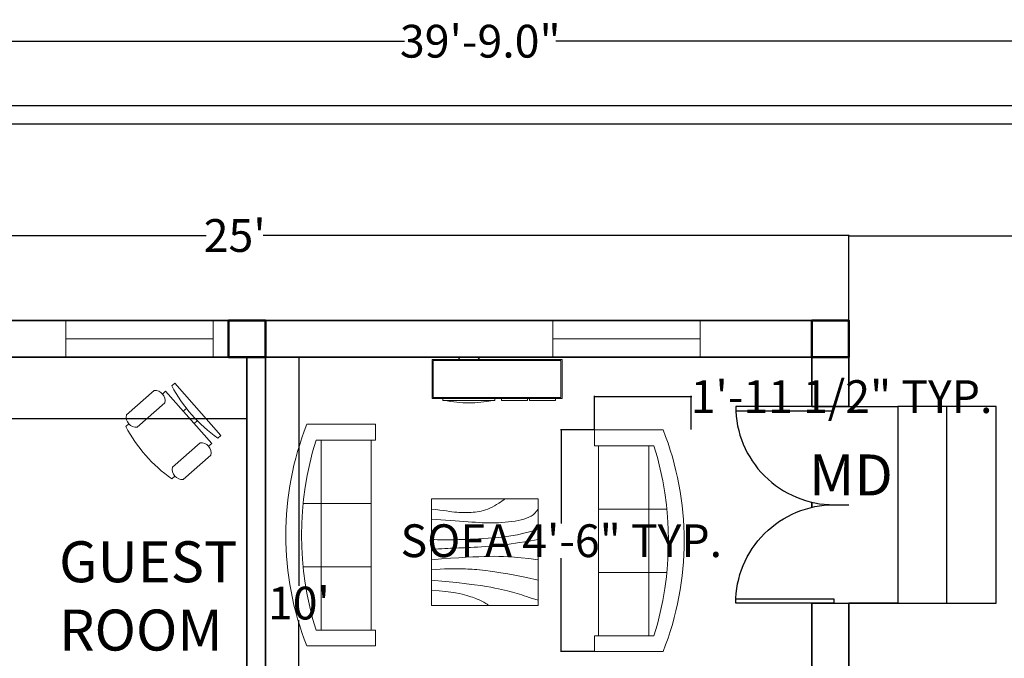
# Model space of a CAD drawing. Units: inches. Extents: x 20414 to 21627, y 49019 to 50314.
# Tile 8 of 10: x 20594 to 20835, y 50159 to 50314. Entities that reach past the tile are written whole.
import ezdxf

# ---------------------------------------------------------------- set-up
doc = ezdxf.new("R2010")
doc.units = ezdxf.units.IN
for name, color, linetype, lineweight in [('A-ANNO-DIMS', 7, 'Continuous', 18), ('A-AREA-IDEN', 7, 'Continuous', 18), ('C-PROP', 6, 'Continuous', 25), ('columns', 1, 'Continuous', 50), ('doors', 3, 'Continuous', 25), ('furniture', 2, 'Continuous', 18), ('stairs', 4, 'Continuous', 25), ('text', 3, 'Continuous', 25), ('walls', 6, 'Continuous', 35), ('windows', 3, 'Continuous', 18)]:
    doc.layers.add(name, color=color, linetype=linetype, lineweight=lineweight)
doc.styles.get("Standard").update_dxf_attribs({"font": 'arial.ttf'})
doc.dimstyles.get("Standard").update_dxf_attribs({"dimtxt": 8, "dimasz": 0.18, "dimexe": 0.18, "dimexo": 0.0625, "dimgap": 0.09, "dimtad": 0, "dimtih": 1, "dimtoh": 1, "dimdec": 1, "dimzin": 0, "dimdsep": 46, "dimlunit": 3, "dimtxsty": 'Standard', "dimcen": 0.09, "dimadec": 0, "dimazin": 0, "dimtfac": 1, "dimtdec": 1, "dimtofl": 0, "dimtmove": 0, "dimatfit": 3, "dimfxl": 1, "dimtolj": 1, "dimtzin": 0, "dimarcsym": 0})

# ---------------------------------------------------------------- blocks, each defined once
blk = doc.blocks.new('Table - Square Woodgrain 42 x 42 in.')
blk.add_line((0, -42), (42, -42))
for points in [[(0, -4), (1.704, -4.2172), (3.2358, -4.4188), (4.615, -4.604), (5.8615, -4.7721), (6.9951, -4.9224), (8.0357, -5.0541), (9.0031, -5.1667), (9.9171, -5.2594), (10.7951, -5.3316), (11.6445, -5.3836), (12.4702, -5.4157), (13.277, -5.4283), (14.0698, -5.4217), (14.8535, -5.3964), (15.6331, -5.3526), (16.4133, -5.2908), (17.1986, -5.2103), (17.9913, -5.1062), (18.793, -4.9727), (19.6056, -4.8038), (20.4307, -4.5937), (21.2701, -4.3365), (22.1256, -4.0262), (22.9989, -3.6571), (23.888, -3.2272), (24.7756, -2.7516), (25.6408, -2.2491), (26.4624, -1.7387), (27.2195, -1.2395), (27.891, -0.7703), (28.456, -0.3501), (28.8934, 0.002)], [(0, -42), (0, 0), (42, 0), (42, -42)], [(0, -8), (1.8203, -8.1001), (3.6741, -8.2149), (5.5411, -8.3408), (7.4011, -8.4741), (9.2339, -8.6112), (11.0193, -8.7484), (12.7371, -8.8821), (14.3671, -9.0086), (15.8954, -9.1246), (17.3337, -9.2278), (18.6997, -9.3159), (20.0116, -9.387), (21.2871, -9.4389), (22.5442, -9.4696), (23.8008, -9.477), (25.0749, -9.459), (26.3791, -9.4137), (27.7049, -9.3403), (29.0383, -9.2382), (30.3655, -9.1068), (31.6728, -8.9455), (32.9461, -8.7535), (34.1717, -8.5304), (35.3358, -8.2756), (36.4268, -7.9863), (37.443, -7.6521), (38.3849, -7.2603), (39.253, -6.7986), (40.048, -6.2542), (40.7705, -5.6147), (41.421, -4.8674), (42, -4)], [(42, -12), (39.1784, -12.8621), (36.4519, -13.5654), (33.8246, -14.1294), (31.3004, -14.5731), (28.8832, -14.9161), (26.577, -15.1775), (24.3858, -15.3768), (22.3136, -15.5332), (20.3622, -15.6632), (18.5254, -15.7718), (16.7947, -15.8612), (15.1618, -15.9338), (13.6183, -15.9916), (12.1558, -16.0369), (10.7659, -16.0718), (9.4403, -16.0987), (8.1703, -16.1191), (6.9461, -16.1325), (5.7577, -16.1377), (4.595, -16.1335), (3.4479, -16.1188), (2.3064, -16.0924), (1.1604, -16.0532), (0, -16)], [(42, -16), (37.6529, -16.7365), (33.8802, -17.329), (30.6179, -17.7961), (27.8015, -18.1561), (25.3668, -18.4275), (23.2497, -18.6288), (21.3859, -18.7785), (19.7111, -18.8949), (18.1693, -18.9939), (16.7375, -19.0795), (15.401, -19.1534), (14.1449, -19.217), (12.9544, -19.2717), (11.8148, -19.3191), (10.7113, -19.3606), (9.6291, -19.3976), (8.5534, -19.4323), (7.47, -19.4689), (6.3643, -19.5122), (5.222, -19.5672), (4.0288, -19.6386), (2.7703, -19.7313), (1.4321, -19.8501), (0, -20)], [(0, -24), (3.9243, -23.6805), (7.4766, -23.4138), (10.6891, -23.1954), (13.5943, -23.0205), (16.2247, -22.8847), (18.6125, -22.7832), (20.7903, -22.7116), (22.7903, -22.6651), (24.6563, -22.642), (26.4764, -22.6507), (28.35, -22.7024), (30.3766, -22.8084), (32.6555, -22.98), (35.2861, -23.2283), (38.3678, -23.5645), (42, -24)], [(42, -32), (37.392, -31.017), (33.4585, -30.2231), (30.1291, -29.5949), (27.3334, -29.109), (25.0009, -28.742), (23.0612, -28.4707), (21.4439, -28.2716), (20.0786, -28.1215), (18.8998, -28.0002), (17.8609, -27.9014), (16.9206, -27.8219), (16.0371, -27.7588), (15.1691, -27.709), (14.2748, -27.6693), (13.3128, -27.6368), (12.2415, -27.6083), (11.0295, -27.5824), (9.6867, -27.5643), (8.233, -27.5608), (6.6884, -27.5787), (5.0728, -27.6248), (3.4062, -27.7058), (1.7086, -27.8286), (0, -28)], [(0, -32), (5.4026, -32.5358), (9.9494, -33.019), (13.7424, -33.4553), (16.8834, -33.8505), (19.4743, -34.2106), (21.6171, -34.5413), (23.4136, -34.8486), (24.9657, -35.1382), (26.3614, -35.4156), (27.6332, -35.6841), (28.7995, -35.9467), (29.8788, -36.2064), (30.8897, -36.4661), (31.8507, -36.7288), (32.7802, -36.9973), (33.6968, -37.2747), (34.6175, -37.5635), (35.5531, -37.8651), (36.5128, -38.1805), (37.506, -38.5108), (38.5421, -38.8568), (39.6302, -39.2197), (40.7797, -39.6004), (42, -40)], [(0, -36), (3.0098, -36.2857), (5.5354, -36.5643), (7.6368, -36.8359), (9.374, -37.1009), (10.807, -37.3597), (11.9957, -37.6126), (13.0002, -37.8599), (13.8804, -38.102), (14.6874, -38.3393), (15.4365, -38.5729), (16.1338, -38.8041), (16.7858, -39.0341), (17.3987, -39.264), (17.9787, -39.4952), (18.5322, -39.7288), (19.0655, -39.9662), (19.5832, -40.2081), (20.0842, -40.4544), (20.5657, -40.7046), (21.0249, -40.9581), (21.459, -41.2144), (21.8653, -41.4731), (22.2409, -41.7335), (22.5831, -41.9951)]]:
    blk.add_lwpolyline(points)
blk = doc.blocks.new('Sofa - Roundback 7 ft.')
for p, q in [((-12.00002, -32.4421), (-12.00003, -6.5971)), ((11.99997, -32.4421), (11.99998, -6.5971)), ((-36.000027, -34), (-36.000027, -11.4696)), ((-35.999844, -13.3819), (35.9998, -13.3819)), ((35.99998, -34), (35.99998, -11.4696)), ((-36.000027, -32.4421), (35.99998, -32.4421))]:
    blk.add_line(p, q)
for points in [[(-36.000027, -34), (-42.000027, -34), (-42.000027, -8)], [(41.99998, -8), (41.99998, -34), (35.99998, -34)]]:
    blk.add_lwpolyline(points)
for centre, radius, start, end in [((0, -114.25), 114.25, 68.43141, 111.5686), ((-0.00001, -127.1968), 121.1968, 72.72033, 107.2797)]:
    blk.add_arc(centre, radius, start, end)
blk = doc.blocks.new('*U14')
for p, q in [((0, 0), (0, 6)), ((40, 0), (40, 6))]:
    blk.add_line(p, q)
blk.add_lwpolyline([(0, 0), (0, -40), (1.75, -40), (1.75, 0)], close=True)
blk.add_arc((0, 0), 40, 270, 0)
blk = doc.blocks.new('Entertainment Center')
for p, q in [((-4, 0), (-5, -1)), ((4, 0), (-4, 0)), ((5, -1), (4, 0)), ((-17, -19), (-17, -1)), ((-17, -1), (43, -1)), ((-16.5, -18.5), (-16.5, -1.5)), ((-16.5, -1.5), (42.5, -1.5)), ((42.5, -1.5), (42.5, -18.5)), ((43, -1), (43, -19)), ((43, -19), (-17, -19)), ((42.5, -18.5), (-16.5, -18.5)), ((-12, -20), (-12, -19)), ((12, -20), (-12, -20)), ((12, -19), (12, -20)), ((15, -20), (15, -19)), ((27, -20), (15, -20)), ((27, -19), (27, -20)), ((28, -20), (28, -19)), ((40, -20), (28, -20)), ((40, -19), (40, -20))]:
    blk.add_line(p, q)
blk.add_arc((0, 40), 61, 259.6111, 280.3889)
blk = doc.blocks.new('Chair - Desk')
for p, q in [((-8.5, 0), (-8.5, -1)), ((-8.5, 0), (8.5, 0)), ((8.5, 0), (8.5, -1)), ((-2, -3), (-2, -1.9355)), ((2, -1.9576), (2, -3)), ((-8.5, -3), (-8.5, -4)), ((-8.5, -3), (8.5, -3)), ((8.5, -3), (8.5, -4)), ((-10.5, -5), (-10.5, -14)), ((-6.5, -14), (-6.5, -5)), ((6.5, -5), (6.5, -14)), ((10.5, -14), (10.5, -5)), ((-8.5, -15), (-8.5, -16)), ((8.5, -15), (8.5, -16))]:
    blk.add_line(p, q)
for centre, radius, start, end in [((0, 34.625), 36.625, 256.5803, 283.4197), ((-8.5, -6.5), 2.5, 36.8699, 143.1301), ((8.5, -6.5), 2.5, 36.8699, 143.1301), ((-8.5, -12.5), 2.5, 216.8699, 323.1301), ((8.5, -12.5), 2.5, 216.8699, 323.1301), ((0, 19.625), 36.625, 256.5803, 283.4197)]:
    blk.add_arc(centre, radius, start, end)
blk = doc.blocks.new('*D29')
at = {"layer": 'A-ANNO-DIMS', "color": 0, "lineweight": -2, "transparency": 16777216}
for p, q in [((20506.01, 50219.94), (20506.01, 50216.8)), ((20649.99, 50219.94), (20649.99, 50216.8)), ((20506.19, 50216.98), (20571.5, 50216.98)), ((20649.81, 50216.98), (20584.5, 50216.98))]:
    blk.add_line(p, q, dxfattribs=at)
at = {"layer": 'A-ANNO-DIMS', "color": 0, "transparency": 16777216}
for points in [[(20506.19, 50217.01), (20506.19, 50216.95), (20506.01, 50216.98)], [(20649.81, 50217.01), (20649.81, 50216.95), (20649.99, 50216.98)]]:
    blk.add_solid(points, dxfattribs=at)
at = {"layer": 'Defpoints', "color": 0, "transparency": 16777216}
for p in [(20506.01, 50220.01), (20649.99, 50220.01), (20649.99, 50216.98)]:
    blk.add_point(p, dxfattribs=at)
at = {"layer": 'A-ANNO-DIMS', "color": 0, "transparency": 16777216, "insert": (20578, 50216.98), "char_height": 8, "attachment_point": 5}
blk.add_mtext("\\A1;12'", dxfattribs=at)
blk = doc.blocks.new('*D30')
at = {"layer": 'A-ANNO-DIMS', "color": 0, "lineweight": -2, "transparency": 16777216}
for p, q in [((20497.01, 50241.07), (20497.01, 50261.92)), ((20497.19, 50261.74), (20640.05, 50261.74)), ((20796.81, 50261.74), (20653.95, 50261.74)), ((20796.99, 50241.07), (20796.99, 50261.92))]:
    blk.add_line(p, q, dxfattribs=at)
at = {"layer": 'A-ANNO-DIMS', "color": 0, "transparency": 16777216}
for points in [[(20497.19, 50261.77), (20497.19, 50261.71), (20497.01, 50261.74)], [(20796.81, 50261.77), (20796.81, 50261.71), (20796.99, 50261.74)]]:
    blk.add_solid(points, dxfattribs=at)
at = {"layer": 'Defpoints', "color": 0, "transparency": 16777216}
for p in [(20796.99, 50261.74), (20497.01, 50241.01), (20796.99, 50241.01)]:
    blk.add_point(p, dxfattribs=at)
at = {"layer": 'A-ANNO-DIMS', "color": 0, "transparency": 16777216, "insert": (20647, 50261.74), "char_height": 8, "attachment_point": 5}
blk.add_mtext("\\A1;25'", dxfattribs=at)
blk = doc.blocks.new('*D51')
at = {"layer": 'A-ANNO-DIMS', "color": 0, "lineweight": -2, "transparency": 16777216}
for p, q in [((20654.55, 50232.01), (20662.87, 50232.01)), ((20662.69, 50231.83), (20662.69, 50176.18)), ((20662.69, 50112.19), (20662.69, 50167.83)), ((20654.55, 50112.01), (20662.87, 50112.01))]:
    blk.add_line(p, q, dxfattribs=at)
at = {"layer": 'A-ANNO-DIMS', "color": 0, "transparency": 16777216}
for points in [[(20662.66, 50231.83), (20662.72, 50231.83), (20662.69, 50232.01)], [(20662.66, 50112.19), (20662.72, 50112.19), (20662.69, 50112.01)]]:
    blk.add_solid(points, dxfattribs=at)
at = {"layer": 'Defpoints', "color": 0, "transparency": 16777216}
for p in [(20654.49, 50232.01), (20654.49, 50112.01), (20662.69, 50112.01)]:
    blk.add_point(p, dxfattribs=at)
at = {"layer": 'A-ANNO-DIMS', "color": 0, "transparency": 16777216, "insert": (20662.69, 50172.01), "char_height": 8, "attachment_point": 5}
blk.add_mtext("\\A1;10'", dxfattribs=at)
blk = doc.blocks.new('*D59')
at = {"layer": 'A-ANNO-DIMS', "color": 0, "lineweight": -2, "transparency": 16777216}
for p, q in [((20796.99, 50241.07), (20796.99, 50261.82)), ((20797.17, 50261.64), (20862.49, 50261.64)), ((20940.81, 50261.64), (20875.49, 50261.64)), ((20940.99, 50241.07), (20940.99, 50261.82))]:
    blk.add_line(p, q, dxfattribs=at)
at = {"layer": 'A-ANNO-DIMS', "color": 0, "transparency": 16777216}
for points in [[(20797.17, 50261.67), (20797.17, 50261.61), (20796.99, 50261.64)], [(20940.81, 50261.67), (20940.81, 50261.61), (20940.99, 50261.64)]]:
    blk.add_solid(points, dxfattribs=at)
at = {"layer": 'Defpoints', "color": 0, "transparency": 16777216}
for p in [(20940.99, 50261.64), (20796.99, 50241.01), (20940.99, 50241.01)]:
    blk.add_point(p, dxfattribs=at)
at = {"layer": 'A-ANNO-DIMS', "color": 0, "transparency": 16777216, "insert": (20868.99, 50261.64), "char_height": 8, "attachment_point": 5}
blk.add_mtext("\\A1;12'", dxfattribs=at)
blk = doc.blocks.new('*D61')
at = {"layer": 'A-ANNO-DIMS', "color": 0, "lineweight": -2, "transparency": 16777216}
for p, q in [((20468.49, 50293.57), (20468.49, 50309.35)), ((20468.67, 50309.17), (20688.5, 50309.17)), ((20945.31, 50309.17), (20725.48, 50309.17)), ((20945.49, 50293.57), (20945.49, 50309.35))]:
    blk.add_line(p, q, dxfattribs=at)
at = {"layer": 'A-ANNO-DIMS', "color": 0, "transparency": 16777216}
for points in [[(20468.67, 50309.2), (20468.67, 50309.14), (20468.49, 50309.17)], [(20945.31, 50309.2), (20945.31, 50309.14), (20945.49, 50309.17)]]:
    blk.add_solid(points, dxfattribs=at)
at = {"layer": 'Defpoints', "color": 0, "transparency": 16777216}
for p in [(20945.49, 50309.17), (20468.49, 50293.51), (20945.49, 50293.51)]:
    blk.add_point(p, dxfattribs=at)
at = {"layer": 'A-ANNO-DIMS', "color": 0, "transparency": 16777216, "insert": (20706.99, 50309.17), "char_height": 8, "attachment_point": 5}
blk.add_mtext('\\A1;39\'-9.0"', dxfattribs=at)
blk = doc.blocks.new('WINDOW-36IN-PLAN')
for p, q in [((9, 36), (0, 36)), ((4.5, 36), (4.5, 0)), ((9, 0), (0, 0))]:
    blk.add_line(p, q)
blk = doc.blocks.new('COLUMN-9X9')
blk.add_lwpolyline([(0, 9), (0, 0), (9, 0), (9, 9), (0, 9)])
blk = doc.blocks.new('*D82')
at = {"layer": 'A-ANNO-DIMS', "color": 0, "lineweight": -2, "transparency": 16777216}
for p, q in [((20734.84, 50214.29), (20726.6, 50214.29)), ((20726.78, 50214.11), (20726.78, 50191.46)), ((20726.78, 50160.36), (20726.78, 50183)), ((20734.84, 50160.18), (20726.6, 50160.18))]:
    blk.add_line(p, q, dxfattribs=at)
at = {"layer": 'A-ANNO-DIMS', "color": 0, "transparency": 16777216}
for points in [[(20726.75, 50214.11), (20726.81, 50214.11), (20726.78, 50214.29)], [(20726.75, 50160.36), (20726.81, 50160.36), (20726.78, 50160.18)]]:
    blk.add_solid(points, dxfattribs=at)
at = {"layer": 'Defpoints', "color": 0, "transparency": 16777216}
for p in [(20726.78, 50214.29), (20734.9, 50214.29), (20734.9, 50160.18)]:
    blk.add_point(p, dxfattribs=at)
at = {"layer": 'A-ANNO-DIMS', "color": 0, "transparency": 16777216, "insert": (20726.78, 50187.23), "char_height": 8, "attachment_point": 5}
blk.add_mtext('\\A1;SOFA 4\'-6" TYP.', dxfattribs=at)
blk = doc.blocks.new('*D83')
at = {"layer": 'A-ANNO-DIMS', "color": 0, "lineweight": -2, "transparency": 16777216}
for p, q in [((20734.9, 50214.35), (20734.9, 50222.59)), ((20735.08, 50222.41), (20758.34, 50222.41)), ((20758.52, 50214.35), (20758.52, 50222.59)), ((20758.52, 50222.41), (20758.7, 50222.41))]:
    blk.add_line(p, q, dxfattribs=at)
at = {"layer": 'A-ANNO-DIMS', "color": 0, "transparency": 16777216}
for points in [[(20735.08, 50222.44), (20735.08, 50222.38), (20734.9, 50222.41)], [(20758.34, 50222.44), (20758.34, 50222.38), (20758.52, 50222.41)]]:
    blk.add_solid(points, dxfattribs=at)
at = {"layer": 'Defpoints', "color": 0, "transparency": 16777216}
for p in [(20758.52, 50222.41), (20734.9, 50214.29), (20758.52, 50214.29)]:
    blk.add_point(p, dxfattribs=at)
at = {"layer": 'A-ANNO-DIMS', "color": 0, "transparency": 16777216, "insert": (20795.23, 50222.41), "char_height": 8, "attachment_point": 5}
blk.add_mtext('\\A1;1\'-11 1/2" TYP.', dxfattribs=at)

msp = doc.modelspace()

# ---------------------------------------------------------------- linework, layer by layer
at = {"layer": 'C-PROP'}
for p, q in [((20468.49, 50293.51), (20945.49, 50293.51)), ((20472.99, 50289.01), (20940.99, 50289.01))]:
    msp.add_line(p, q, dxfattribs=at)
at = {"layer": 'doors'}
for p, q in [((20787.99, 50220.01), (20796.99, 50220.01)), ((20796.99, 50220.01), (20787.99, 50220.01)), ((20787.99, 50172.01), (20796.99, 50172.01)), ((20787.99, 50172.01), (20796.99, 50172.01))]:
    msp.add_line(p, q, dxfattribs=at)
at = {"layer": 'stairs'}
for points in [[(20796.99, 50220.01), (20808.99, 50220.01), (20808.99, 50172.01), (20796.99, 50172.01), (20820.99, 50172.01), (20820.99, 50220.01), (20808.99, 50220.01)], [(20820.99, 50172.01), (20832.99, 50172.01), (20832.99, 50220.01), (20820.99, 50220.01)]]:
    msp.add_lwpolyline(points, dxfattribs=at)
at = {"layer": 'walls'}
for p, q in [((20496.99, 50241.01), (20796.99, 50241.01)), ((20796.99, 50241.01), (20796.99, 50220.01)), ((20505.99, 50232.01), (20649.99, 50232.01)), ((20649.99, 50112.01), (20649.99, 50232.01)), ((20654.49, 50103.01), (20654.49, 50232.01)), ((20654.49, 50232.01), (20787.99, 50232.01)), ((20787.99, 50232.01), (20787.99, 50220.01)), ((20787.99, 50196.62), (20787.99, 50195.39)), ((20787.99, 50172.01), (20787.99, 50107.51)), ((20796.99, 50172.01), (20796.99, 49821.01))]:
    msp.add_line(p, q, dxfattribs=at)

# ---------------------------------------------------------------- block references
at = {"layer": 'columns'}
for p in [(20645.49, 50232.01), (20787.99, 50232.01)]:
    msp.add_blockref('COLUMN-9X9', p, dxfattribs=at)
at = {"layer": 'doors', "yscale": 0.6, "zscale": 0.6, "rotation": 270}
for p, xscale in [((20793.39, 50220.01), 0.6), ((20793.39, 50172.01), -0.6)]:
    msp.add_blockref('*U14', p, dxfattribs=dict(at, xscale=xscale))
at = {"layer": 'furniture'}
for name, p, xscale, yscale, zscale in [('Entertainment Center', (20704.2, 50232.01), 0.5294023735262411, 0.5294023735262411, 0.5294023735262411), ('Table - Square Woodgrain 42 x 42 in.', (20695.1, 50197.44), 0.6190476190476191, 0.6190476190476191, 0.6190476190476191)]:
    msp.add_blockref(name, p, dxfattribs=dict(at, xscale=xscale, yscale=yscale, zscale=zscale))
at = {"layer": 'furniture', "rotation": 311.4332562192998}
msp.add_blockref('Chair - Desk', (20638, 50219.32), dxfattribs=at)
at = {"layer": 'furniture', "yscale": 0.6442431863649634, "zscale": 0.6442431863649634}
for p, xscale, rotation in [((20659.47, 50188.59), 0.6442431863649634, 90), ((20756.8, 50187.23), -0.6442431863649634, 270)]:
    msp.add_blockref('Sofa - Roundback 7 ft.', p, dxfattribs=dict(at, xscale=xscale, rotation=rotation))
at = {"layer": 'windows'}
for p, rotation in [((20605.78, 50241.01), 270.0000000000218), ((20724.73, 50241.01), 270.0000000000245)]:
    msp.add_blockref('WINDOW-36IN-PLAN', p, dxfattribs=dict(at, rotation=rotation))

# ---------------------------------------------------------------- texts
at = {"layer": 'A-AREA-IDEN', "insert": (20604.1, 50187.09), "char_height": 10, "attachment_point": 1}
msp.add_mtext_dynamic_manual_height_columns('GUEST\\PROOM', width=44.4717, gutter_width=50, heights=[34.97], dxfattribs=at)
at = {"layer": 'text', "insert": (20787.3, 50208.28), "char_height": 10, "attachment_point": 1}
msp.add_mtext_dynamic_manual_height_columns('MD', width=44.4717, gutter_width=50, heights=[34.97], dxfattribs=at)

# ---------------------------------------------------------------- dimensions: what is measured, and where the dimension line sits
at = {"layer": 'A-ANNO-DIMS'}
for base, p1, p2, picture, middle in [((20945.49, 50309.17), (20468.49, 50293.51), (20945.49, 50293.51), '*D61', (20706.99, 50309.17)), ((20796.99, 50261.74), (20497.01, 50241.01), (20796.99, 50241.01), '*D30', (20647, 50261.74)), ((20940.99, 50261.64), (20796.99, 50241.01), (20940.99, 50241.01), '*D59', (20868.99, 50261.64)), ((20649.99, 50216.98), (20506.01, 50220.01), (20649.99, 50220.01), '*D29', (20578, 50216.98))]:
    dim = msp.add_linear_dim(base=base, p1=p1, p2=p2, dimstyle='Standard', override={"dimclrd": 0, "dimclre": 0, "dimclrt": 0}, dxfattribs=at)
    dim.commit()
    dim.dimension.update_dxf_attribs({"geometry": picture, "text_midpoint": middle})
dim = msp.add_linear_dim(base=(20758.52, 50222.41), p1=(20734.9, 50214.29), p2=(20758.52, 50214.29), text='<> TYP.', dimstyle='Standard', override={"dimdec": 1, "dimlfac": 1, "dimrnd": 0, "dimzin": 1, "dimdsep": 46, "dimlunit": 4, "dimfrac": 2}, dxfattribs=at)
dim.commit()
dim.dimension.update_dxf_attribs({"geometry": '*D83', "text_midpoint": (20795.23, 50222.41)})
dim = msp.add_linear_dim(base=(20662.69, 50112.01), p1=(20654.49, 50232.01), p2=(20654.49, 50112.01), angle=90, dimstyle='Standard', override={"dimclrd": 0, "dimclre": 0, "dimclrt": 0}, dxfattribs=at)
dim.commit()
dim.dimension.update_dxf_attribs({"geometry": '*D51', "text_midpoint": (20662.69, 50172.01)})
dim = msp.add_linear_dim(base=(20726.78, 50214.29), p1=(20734.9, 50160.18), p2=(20734.9, 50214.29), angle=90, text='SOFA <> TYP.', dimstyle='Standard', override={"dimdec": 1, "dimlfac": 1, "dimrnd": 0, "dimzin": 1, "dimdsep": 46, "dimlunit": 4, "dimfrac": 2}, dxfattribs=at)
dim.commit()
dim.dimension.update_dxf_attribs({"geometry": '*D82', "text_midpoint": (20726.78, 50187.23)})

doc.saveas('drawing.dxf')
